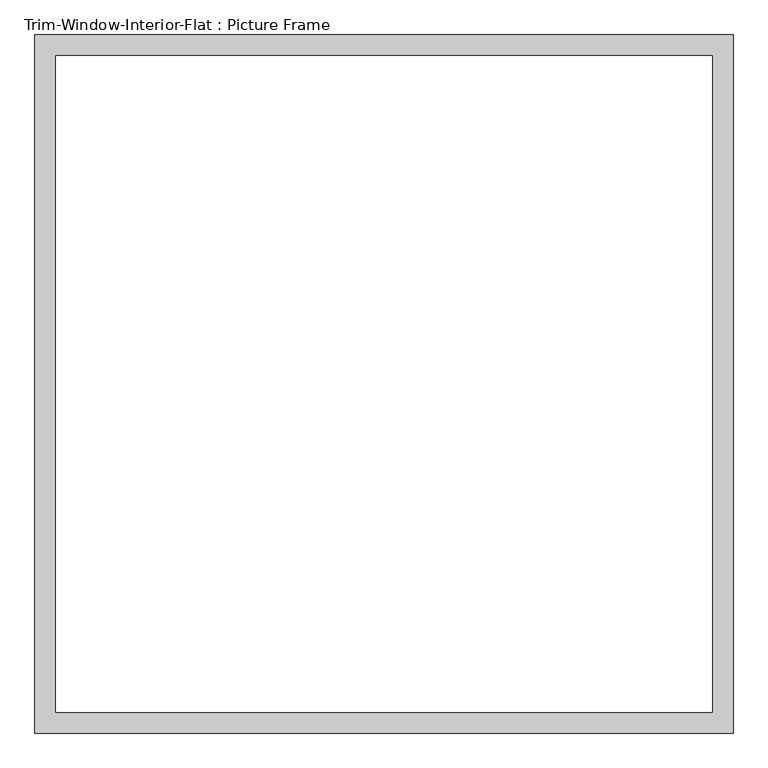
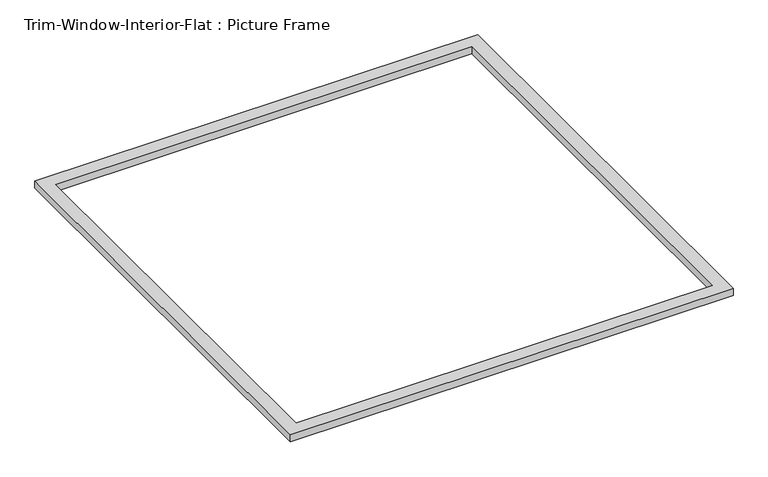
"""IFC4 building model written with IfcOpenShell, lengths in millimetres: proxy geometry, Trim-Window-Interior-Flat : Picture Frame."""

from ifc_helpers import new_model, si_unit, origin, origin_with_axes, place, context, project, spatial, polyline, outline, extrude, source, transform, mapped, element, save


def trim_window_interior_flat_picture_frame_bfefb25c(model_context):
    return source(origin(), model_context, "Body", "SweptSolid", [
        extrude(outline(polyline([(958.85, 44.45), (958.85, -1873.25), (-958.85, -1873.25), (-958.85, 44.45), (958.85, 44.45)]), holes=[polyline([(901.7, -12.7), (-901.7, -12.7), (-901.7, -1816.1), (901.7, -1816.1), (901.7, -12.7)])]), origin_with_axes(), (0.0, 0.0, 1.0), 31.75),
    ])


if __name__ == "__main__":
    model = new_model("IFC4")
    model_context = context("Model", 3, world=origin())
    ifc_project = project(units=[si_unit("LENGTHUNIT", "METRE", prefix="MILLI")], contexts=[model_context])
    site = spatial("IfcSite", under=ifc_project)
    building = spatial("IfcBuilding", under=site)
    placement = place(None, origin())
    trim_window_interior_flat_picture_frame_shape = trim_window_interior_flat_picture_frame_bfefb25c(model_context)
    element("IfcBuildingElementProxy", 1, Name="Trim-Window-Interior-Flat : Picture Frame", ObjectType="Trim-Window-Interior-Flat : Picture Frame", at=placement, inside=building, context=model_context, shape_type="MappedRepresentation", body=[
        mapped(trim_window_interior_flat_picture_frame_shape, transform((0.0, 0.0, 0.0), x_axis=(1.0, 0.0, 0.0), y_axis=(0.0, 1.0, 0.0), z_axis=(0.0, 0.0, 1.0))),
    ])
    save(model, "model.ifc")

# Revit data of these elements
# Type "Trim-Window-Interior-Flat : Picture Frame"
#   Trim Thickness_Picture Frame = 0' - 1 1/4"
#   Trim Width = 0' - 2 1/4"
#   Trim Thickness_with Sill = 0' - 0 3/4"
#   Sill Thickness = 0' - 1 1/4"
#   Opening Width [instance default] = 2' - 0"
#   Opening Height [instance default] = 3' - 0"
#   Default Elevation = 4' - 0"
#   Sill = no
#   Picture Frame = yes
#   Trim Material [instance default] = none
# Element 1 (IfcBuildingElementProxy, "Trim-Window-Interior-Flat : Picture Frame")
#   Opening Width = 6' - 0"
#   Opening Height = 6' - 0"
#   Trim Material = Wood - Stained
#   Materials on its faces: "Wood - Stained"
# Materials
#   "Wood - Stained": class "Wood", colour RGB 224 178 126, transparency 0, Cost = 0
